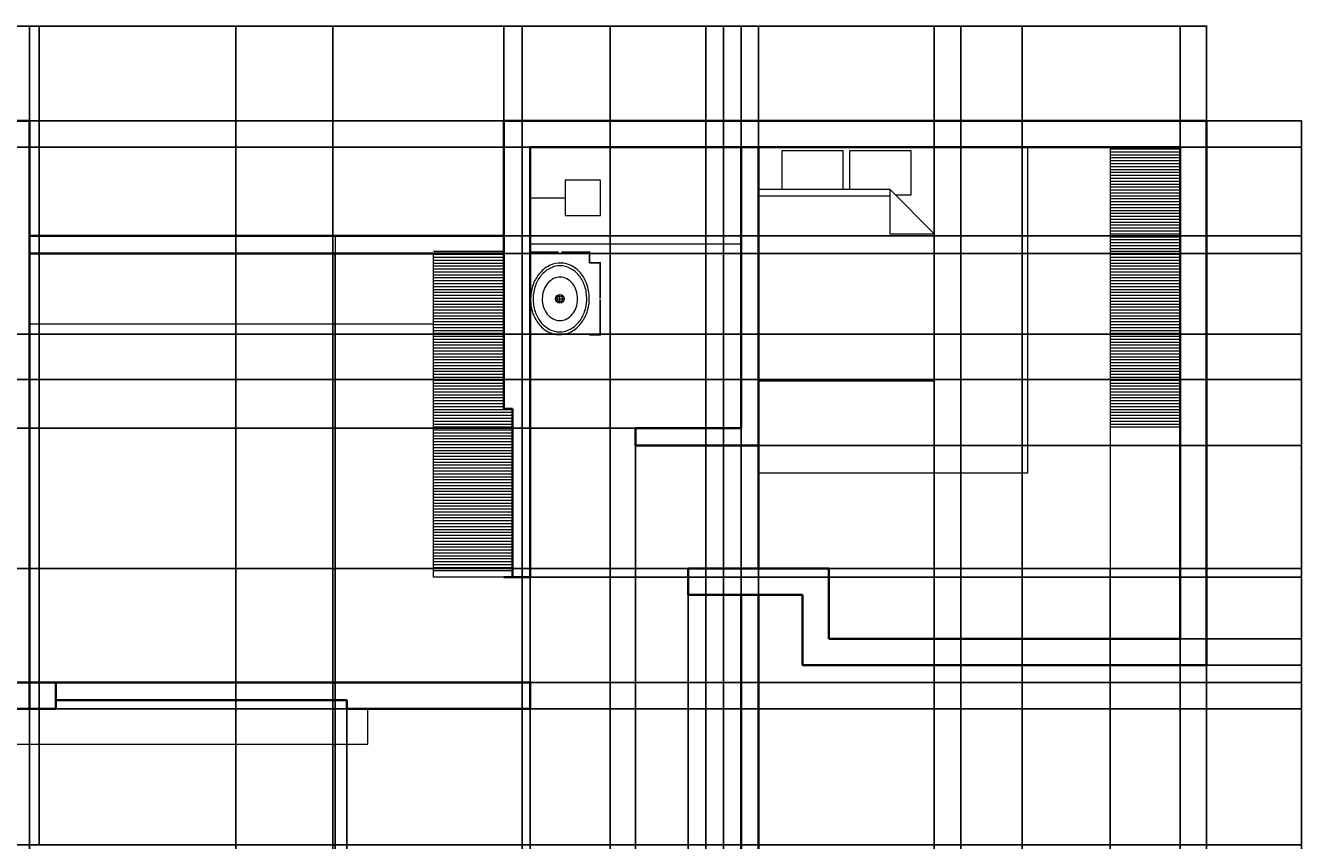
# Model space of a CAD drawing. Units: inches. Extents: x 1159 to 1869, y 2212 to 2738.
# Tile 5 of 5: x 1433 to 1869, y 2460 to 2738. Entities that reach past the tile are written whole.
import ezdxf

# ---------------------------------------------------------------- set-up
doc = ezdxf.new("R2010")
doc.units = ezdxf.units.IN
for name, color, linetype, lineweight in [('A-ANNO-DIMS', 2, 'Continuous', 18), ('A-FLOR', 9, 'Continuous', 13), ('A-FLOR-CASE', 30, 'Continuous', 18), ('A-FLOR-FIXT', 9, 'Continuous', 18), ('A-FLOR-PATT', 252, 'Continuous', 13), ('A-FURN', 8, 'Continuous', 18), ('A-GLAZ', 4, 'Continuous', 18), ('A-WALL', 7, 'Continuous', 35)]:
    doc.layers.add(name, color=color, linetype=linetype, lineweight=lineweight)
doc.styles.get("Standard").update_dxf_attribs({"font": 'arial.ttf'})
doc.dimstyles.get("Standard").update_dxf_attribs({"dimtxt": 0.18, "dimasz": 0.18, "dimexe": 0.18, "dimexo": 0.0625, "dimgap": 0.09, "dimtad": 0, "dimtih": 1, "dimtoh": 1, "dimdec": 4, "dimzin": 0, "dimdsep": 46, "dimtxsty": 'Standard', "dimcen": 0.09, "dimadec": 0, "dimazin": 0, "dimtfac": 1, "dimtdec": 4, "dimtofl": 0, "dimtmove": 0, "dimatfit": 3, "dimfxl": 1, "dimtolj": 1, "dimtzin": 0, "dimarcsym": 0})

# ---------------------------------------------------------------- blocks, each defined once
blk = doc.blocks.new('Bed - Queen')
for p, q in [((0, -80.00003), (0, 0)), ((0, 0), (59.99999, 0)), ((59.99999, 0), (59.99999, -80.00003)), ((7.99999, -1.2), (28.79998, -1.2)), ((7.99999, -14.4), (7.99999, -1.2)), ((28.79998, -1.2), (28.79998, -14.4)), ((31.19999, -1.2), (51.99999, -1.2)), ((31.19999, -14.4), (31.19999, -1.2)), ((51.99999, -1.2), (51.99999, -16.4)), ((0, -14.4), (44.8, -14.4)), ((44.8, -16.8), (0, -16.8)), ((59.99999, -29.6), (44.8, -14.4)), ((44.8, -14.4), (44.8, -29.6)), ((51.99999, -16.4), (46.79936, -16.4)), ((44.8, -29.6), (59.99999, -29.6)), ((59.99999, -80.00003), (0, -80.00003))]:
    blk.add_line(p, q)
blk = doc.blocks.new('Sink - Oval top')
for p, q in [((-1, 0), (1, 0)), ((0, 1), (0, -1))]:
    blk.add_line(p, q)
for points in [[(-12.23, 0.39, 0.117634), (-11.46, -3.36, 0.104469), (-8.88, -6.8, 0.090016), (-5.08, -9.07, 0.08192), (-0.32, -10.02, 0.08192), (4.49, -9.38, 0.090016), (8.42, -7.36, 0.104469), (11.22, -4.09, 0.117634), (12.23, -0.39, 0.117634), (11.46, 3.36, 0.104469), (8.88, 6.8, 0.090016), (5.08, 9.07, 0.08192), (0.32, 10.02, 0.08192), (-4.49, 9.38, 0.090016), (-8.42, 7.36, 0.104469), (-11.22, 4.09, 0.117634)], [(-11.29, 0.16, 0.118622), (-10.52, -3.25, 0.104678), (-8.07, -6.36, 0.089562), (-4.54, -8.37, 0.081185), (-0.13, -9.15, 0.081185), (4.3, -8.49, 0.089562), (7.89, -6.58, 0.104678), (10.42, -3.55, 0.118622), (11.29, -0.16, 0.118622), (10.52, 3.25, 0.104678), (8.07, 6.36, 0.089562), (4.54, 8.37, 0.081185), (0.13, 9.15, 0.081185), (-4.3, 8.49, 0.089562), (-7.89, 6.58, 0.104678), (-10.42, 3.55, 0.118622)], [(-7.42, 0.08, 0.118283), (-6.91, -2.17, 0.104607), (-5.29, -4.21, 0.089718), (-2.97, -5.53, 0.081436), (-0.07, -6.04, 0.081436), (2.84, -5.59, 0.089718), (5.2, -4.33, 0.104607), (6.86, -2.32, 0.118283), (7.42, -0.08, 0.118283), (6.91, 2.17, 0.104607), (5.29, 4.21, 0.089718), (2.97, 5.53, 0.081436), (0.07, 6.04, 0.081436), (-2.84, 5.59, 0.089718), (-5.2, 4.33, 0.104607), (-6.86, 2.32, 0.118283)]]:
    blk.add_lwpolyline(points, format="xyb", close=True)
for radius in [1.5, 1]:
    blk.add_circle((0, 0), radius)
blk = doc.blocks.new('SHOWER-HEAD-SQUARE-12IN')
for p, q in [((6, 12), (0, 12)), ((0, 12), (0, 0)), ((12, 12), (6, 12)), ((12, 0), (12, 12)), ((0, 0), (12, 0))]:
    blk.add_line(p, q)
blk = doc.blocks.new('*D8')
at = {"layer": 'A-ANNO-DIMS', "color": 0, "lineweight": -2, "transparency": 16777216}
for p, q in [((1625.69, 2657.04), (1629.49, 2657.04)), ((1629.31, 2656.86), (1629.31, 2644.95)), ((1629.31, 2632.67), (1629.31, 2644.58)), ((1625.69, 2632.49), (1629.49, 2632.49))]:
    blk.add_line(p, q, dxfattribs=at)
at = {"layer": 'A-ANNO-DIMS', "color": 0, "transparency": 16777216}
for points in [[(1629.28, 2656.86), (1629.34, 2656.86), (1629.31, 2657.04)], [(1629.28, 2632.67), (1629.34, 2632.67), (1629.31, 2632.49)]]:
    blk.add_solid(points, dxfattribs=at)
at = {"layer": 'Defpoints', "color": 0, "transparency": 16777216}
for p in [(1625.62, 2657.04), (1629.31, 2657.04), (1625.62, 2632.49)]:
    blk.add_point(p, dxfattribs=at)
at = {"layer": 'A-ANNO-DIMS', "color": 0, "transparency": 16777216, "insert": (1629.31, 2644.77), "char_height": 0.18, "attachment_point": 5}
blk.add_mtext('\\A1;BASIN 25 TYP.', dxfattribs=at)
blk = doc.blocks.new('*D9')
at = {"layer": 'A-ANNO-DIMS', "color": 0, "lineweight": -2, "transparency": 16777216}
for p, q in [((1605.49, 2657.1), (1605.49, 2660.9)), ((1605.67, 2660.72), (1615.03, 2660.72)), ((1625.44, 2660.72), (1616.09, 2660.72)), ((1625.62, 2657.1), (1625.62, 2660.9))]:
    blk.add_line(p, q, dxfattribs=at)
at = {"layer": 'A-ANNO-DIMS', "color": 0, "transparency": 16777216}
for points in [[(1605.67, 2660.75), (1605.67, 2660.69), (1605.49, 2660.72)], [(1625.44, 2660.75), (1625.44, 2660.69), (1625.62, 2660.72)]]:
    blk.add_solid(points, dxfattribs=at)
at = {"layer": 'Defpoints', "color": 0, "transparency": 16777216}
for p in [(1605.49, 2660.72), (1605.49, 2657.04), (1625.62, 2657.04)]:
    blk.add_point(p, dxfattribs=at)
at = {"layer": 'A-ANNO-DIMS', "color": 0, "transparency": 16777216, "insert": (1615.56, 2660.72), "char_height": 0.18, "attachment_point": 5}
blk.add_mtext('\\A1;20 TYP.', dxfattribs=at)
blk = doc.blocks.new('*D20')
at = {"layer": 'A-ANNO-DIMS', "color": 0, "lineweight": -2, "transparency": 16777216}
for p, q in [((1191.4, 2461.27), (1191.4, 2738.15)), ((1191.58, 2737.97), (1513.61, 2737.97)), ((1836.22, 2737.97), (1514.19, 2737.97)), ((1836.4, 2705.69), (1836.4, 2738.15))]:
    blk.add_line(p, q, dxfattribs=at)
at = {"layer": 'A-ANNO-DIMS', "color": 0, "transparency": 16777216}
for points in [[(1191.58, 2738), (1191.58, 2737.94), (1191.4, 2737.97)], [(1836.22, 2738), (1836.22, 2737.94), (1836.4, 2737.97)]]:
    blk.add_solid(points, dxfattribs=at)
at = {"layer": 'Defpoints', "color": 0, "transparency": 16777216}
for p in [(1836.4, 2737.97), (1836.4, 2705.63), (1191.4, 2461.21)]:
    blk.add_point(p, dxfattribs=at)
at = {"layer": 'A-ANNO-DIMS', "color": 0, "transparency": 16777216, "insert": (1513.9, 2737.97), "char_height": 0.18, "attachment_point": 5}
blk.add_mtext('\\A1;645', dxfattribs=at)
blk = doc.blocks.new('*D21')
at = {"layer": 'A-ANNO-DIMS', "color": 0, "lineweight": -2, "transparency": 16777216}
for p, q in [((1836.46, 2705.63), (1868.92, 2705.63)), ((1868.74, 2705.45), (1868.74, 2475.03)), ((1868.74, 2244.26), (1868.74, 2474.67)), ((1752.46, 2244.08), (1868.92, 2244.08))]:
    blk.add_line(p, q, dxfattribs=at)
at = {"layer": 'A-ANNO-DIMS', "color": 0, "transparency": 16777216}
for points in [[(1868.71, 2705.45), (1868.77, 2705.45), (1868.74, 2705.63)], [(1868.71, 2244.26), (1868.77, 2244.26), (1868.74, 2244.08)]]:
    blk.add_solid(points, dxfattribs=at)
at = {"layer": 'Defpoints', "color": 0, "transparency": 16777216}
for p in [(1836.4, 2705.63), (1868.74, 2705.63), (1752.4, 2244.08)]:
    blk.add_point(p, dxfattribs=at)
at = {"layer": 'A-ANNO-DIMS', "color": 0, "transparency": 16777216, "insert": (1868.74, 2474.85), "char_height": 0.18, "attachment_point": 5}
blk.add_mtext('\\A1;461.55', dxfattribs=at)
blk = doc.blocks.new('*D24')
at = {"layer": 'A-ANNO-DIMS', "color": 0, "lineweight": -2, "transparency": 16777216}
for p, q in [((1434.4, 2666.32), (1434.4, 2738.15)), ((1434.58, 2737.97), (1515.12, 2737.97)), ((1596.22, 2737.97), (1515.68, 2737.97)), ((1596.4, 2666.32), (1596.4, 2738.15))]:
    blk.add_line(p, q, dxfattribs=at)
at = {"layer": 'A-ANNO-DIMS', "color": 0, "transparency": 16777216}
for points in [[(1434.58, 2738), (1434.58, 2737.94), (1434.4, 2737.97)], [(1596.22, 2738), (1596.22, 2737.94), (1596.4, 2737.97)]]:
    blk.add_solid(points, dxfattribs=at)
at = {"layer": 'Defpoints', "color": 0, "transparency": 16777216}
for p in [(1596.4, 2737.97), (1434.4, 2666.26), (1596.4, 2666.26)]:
    blk.add_point(p, dxfattribs=at)
at = {"layer": 'A-ANNO-DIMS', "color": 0, "transparency": 16777216, "insert": (1515.4, 2737.97), "char_height": 0.18, "attachment_point": 5}
blk.add_mtext('\\A1;162', dxfattribs=at)
blk = doc.blocks.new('*D25')
at = {"layer": 'A-ANNO-DIMS', "color": 0, "lineweight": -2, "transparency": 16777216}
for p, q in [((1683.4, 2552.69), (1683.4, 2738.15)), ((1683.58, 2737.97), (1755.12, 2737.97)), ((1827.22, 2737.97), (1755.68, 2737.97)), ((1827.4, 2552.69), (1827.4, 2738.15))]:
    blk.add_line(p, q, dxfattribs=at)
at = {"layer": 'A-ANNO-DIMS', "color": 0, "transparency": 16777216}
for points in [[(1683.58, 2738), (1683.58, 2737.94), (1683.4, 2737.97)], [(1827.22, 2738), (1827.22, 2737.94), (1827.4, 2737.97)]]:
    blk.add_solid(points, dxfattribs=at)
at = {"layer": 'Defpoints', "color": 0, "transparency": 16777216}
for p in [(1827.4, 2737.97), (1683.4, 2552.63), (1827.4, 2552.63)]:
    blk.add_point(p, dxfattribs=at)
at = {"layer": 'A-ANNO-DIMS', "color": 0, "transparency": 16777216, "insert": (1755.4, 2737.97), "char_height": 0.18, "attachment_point": 5}
blk.add_mtext('\\A1;144', dxfattribs=at)
blk = doc.blocks.new('*D31')
at = {"layer": 'A-ANNO-DIMS', "color": 0, "lineweight": -2, "transparency": 16777216}
for p, q in [((1698.46, 2519.63), (1868.92, 2519.63)), ((1868.74, 2519.45), (1868.74, 2484.03)), ((1868.74, 2448.26), (1868.74, 2483.67)), ((1683.46, 2448.08), (1868.92, 2448.08))]:
    blk.add_line(p, q, dxfattribs=at)
at = {"layer": 'A-ANNO-DIMS', "color": 0, "transparency": 16777216}
for points in [[(1868.71, 2519.45), (1868.77, 2519.45), (1868.74, 2519.63)], [(1868.71, 2448.26), (1868.77, 2448.26), (1868.74, 2448.08)]]:
    blk.add_solid(points, dxfattribs=at)
at = {"layer": 'Defpoints', "color": 0, "transparency": 16777216}
for p in [(1698.4, 2519.63), (1683.4, 2448.08), (1868.74, 2448.08)]:
    blk.add_point(p, dxfattribs=at)
at = {"layer": 'A-ANNO-DIMS', "color": 0, "transparency": 16777216, "insert": (1868.74, 2483.85), "char_height": 0.18, "attachment_point": 5}
blk.add_mtext('\\A1;71.55', dxfattribs=at)
blk = doc.blocks.new('*D32')
at = {"layer": 'A-ANNO-DIMS', "color": 0, "lineweight": -2, "transparency": 16777216}
for p, q in [((1743.46, 2696.63), (1868.92, 2696.63)), ((1868.74, 2696.45), (1868.74, 2612.81)), ((1868.74, 2528.81), (1868.74, 2612.45)), ((1707.46, 2528.63), (1868.92, 2528.63))]:
    blk.add_line(p, q, dxfattribs=at)
at = {"layer": 'A-ANNO-DIMS', "color": 0, "transparency": 16777216}
for points in [[(1868.71, 2696.45), (1868.77, 2696.45), (1868.74, 2696.63)], [(1868.71, 2528.81), (1868.77, 2528.81), (1868.74, 2528.63)]]:
    blk.add_solid(points, dxfattribs=at)
at = {"layer": 'Defpoints', "color": 0, "transparency": 16777216}
for p in [(1743.4, 2696.63), (1868.74, 2696.63), (1707.4, 2528.63)]:
    blk.add_point(p, dxfattribs=at)
at = {"layer": 'A-ANNO-DIMS', "color": 0, "transparency": 16777216, "insert": (1868.74, 2612.63), "char_height": 0.18, "attachment_point": 5}
blk.add_mtext('\\A1;168', dxfattribs=at)
blk = doc.blocks.new('*D36')
at = {"layer": 'A-ANNO-DIMS', "color": 0, "lineweight": -2, "transparency": 16777216}
for p, q in [((1752.4, 2337.14), (1752.4, 2738.15)), ((1752.58, 2737.97), (1762.7, 2737.97)), ((1773.22, 2737.97), (1763.1, 2737.97)), ((1773.4, 2343.14), (1773.4, 2738.15))]:
    blk.add_line(p, q, dxfattribs=at)
at = {"layer": 'A-ANNO-DIMS', "color": 0, "transparency": 16777216}
for points in [[(1752.58, 2738), (1752.58, 2737.94), (1752.4, 2737.97)], [(1773.22, 2738), (1773.22, 2737.94), (1773.4, 2737.97)]]:
    blk.add_solid(points, dxfattribs=at)
at = {"layer": 'Defpoints', "color": 0, "transparency": 16777216}
for p in [(1773.4, 2737.97), (1773.4, 2343.08), (1752.4, 2337.08)]:
    blk.add_point(p, dxfattribs=at)
at = {"layer": 'A-ANNO-DIMS', "color": 0, "transparency": 16777216, "insert": (1762.9, 2737.97), "char_height": 0.18, "attachment_point": 5}
blk.add_mtext('\\A1;21', dxfattribs=at)
blk = doc.blocks.new('*D37')
at = {"layer": 'A-ANNO-DIMS', "color": 0, "lineweight": -2, "transparency": 16777216}
for p, q in [((1434.46, 2705.63), (1868.92, 2705.63)), ((1868.74, 2705.45), (1868.74, 2686.13)), ((1868.74, 2666.44), (1868.74, 2685.76)), ((1434.46, 2666.26), (1868.92, 2666.26))]:
    blk.add_line(p, q, dxfattribs=at)
at = {"layer": 'A-ANNO-DIMS', "color": 0, "transparency": 16777216}
for points in [[(1868.71, 2705.45), (1868.77, 2705.45), (1868.74, 2705.63)], [(1868.71, 2666.44), (1868.77, 2666.44), (1868.74, 2666.26)]]:
    blk.add_solid(points, dxfattribs=at)
at = {"layer": 'Defpoints', "color": 0, "transparency": 16777216}
for p in [(1434.4, 2705.63), (1868.74, 2705.63), (1434.4, 2666.26)]:
    blk.add_point(p, dxfattribs=at)
at = {"layer": 'A-ANNO-DIMS', "color": 0, "transparency": 16777216, "insert": (1868.74, 2685.94), "char_height": 0.18, "attachment_point": 5}
blk.add_mtext('\\A1;39.37', dxfattribs=at)
blk = doc.blocks.new('*D38')
at = {"layer": 'A-ANNO-DIMS', "color": 0, "lineweight": -2, "transparency": 16777216}
for p, q in [((1434.46, 2660.26), (1868.92, 2660.26)), ((1868.74, 2660.08), (1868.74, 2587.13)), ((1868.74, 2513.81), (1868.74, 2586.76)), ((1443.46, 2513.63), (1868.92, 2513.63))]:
    blk.add_line(p, q, dxfattribs=at)
at = {"layer": 'A-ANNO-DIMS', "color": 0, "transparency": 16777216}
for points in [[(1868.71, 2660.08), (1868.77, 2660.08), (1868.74, 2660.26)], [(1868.71, 2513.81), (1868.77, 2513.81), (1868.74, 2513.63)]]:
    blk.add_solid(points, dxfattribs=at)
at = {"layer": 'Defpoints', "color": 0, "transparency": 16777216}
for p in [(1434.4, 2660.26), (1868.74, 2660.26), (1443.4, 2513.63)]:
    blk.add_point(p, dxfattribs=at)
at = {"layer": 'A-ANNO-DIMS', "color": 0, "transparency": 16777216, "insert": (1868.74, 2586.94), "char_height": 0.18, "attachment_point": 5}
blk.add_mtext('\\A1;146.63', dxfattribs=at)
blk = doc.blocks.new('*D39')
at = {"layer": 'A-ANNO-DIMS', "color": 0, "lineweight": -2, "transparency": 16777216}
for p, q in [((1605.4, 2696.57), (1605.4, 2211.56)), ((1677.4, 2696.57), (1677.4, 2211.56)), ((1605.58, 2211.74), (1641.18, 2211.74)), ((1677.22, 2211.74), (1641.62, 2211.74))]:
    blk.add_line(p, q, dxfattribs=at)
at = {"layer": 'A-ANNO-DIMS', "color": 0, "transparency": 16777216}
for points in [[(1605.58, 2211.77), (1605.58, 2211.71), (1605.4, 2211.74)], [(1677.22, 2211.77), (1677.22, 2211.71), (1677.4, 2211.74)]]:
    blk.add_solid(points, dxfattribs=at)
at = {"layer": 'Defpoints', "color": 0, "transparency": 16777216}
for p in [(1605.4, 2696.63), (1677.4, 2696.63), (1677.4, 2211.74)]:
    blk.add_point(p, dxfattribs=at)
at = {"layer": 'A-ANNO-DIMS', "color": 0, "transparency": 16777216, "insert": (1641.4, 2211.74), "char_height": 0.18, "attachment_point": 5}
blk.add_mtext('\\A1;72', dxfattribs=at)
blk = doc.blocks.new('*D40')
at = {"layer": 'A-ANNO-DIMS', "color": 0, "lineweight": -2, "transparency": 16777216}
for p, q in [((1677.34, 2696.63), (1158.88, 2696.63)), ((1159.06, 2696.45), (1159.06, 2648.81)), ((1159.06, 2600.81), (1159.06, 2648.45)), ((1677.34, 2600.63), (1158.88, 2600.63))]:
    blk.add_line(p, q, dxfattribs=at)
at = {"layer": 'A-ANNO-DIMS', "color": 0, "transparency": 16777216}
for points in [[(1159.03, 2696.45), (1159.09, 2696.45), (1159.06, 2696.63)], [(1159.03, 2600.81), (1159.09, 2600.81), (1159.06, 2600.63)]]:
    blk.add_solid(points, dxfattribs=at)
at = {"layer": 'Defpoints', "color": 0, "transparency": 16777216}
for p in [(1159.06, 2696.63), (1677.4, 2696.63), (1677.4, 2600.63)]:
    blk.add_point(p, dxfattribs=at)
at = {"layer": 'A-ANNO-DIMS', "color": 0, "transparency": 16777216, "insert": (1159.06, 2648.63), "char_height": 0.18, "attachment_point": 5}
blk.add_mtext('\\A1;96', dxfattribs=at)
blk = doc.blocks.new('*D43')
at = {"layer": 'A-ANNO-DIMS', "color": 0, "lineweight": -2, "transparency": 16777216}
for p, q in [((1671.4, 2439.14), (1671.4, 2738.15)), ((1671.58, 2737.97), (1707.18, 2737.97)), ((1743.22, 2737.97), (1707.62, 2737.97)), ((1743.4, 2439.14), (1743.4, 2738.15))]:
    blk.add_line(p, q, dxfattribs=at)
at = {"layer": 'A-ANNO-DIMS', "color": 0, "transparency": 16777216}
for points in [[(1671.58, 2738), (1671.58, 2737.94), (1671.4, 2737.97)], [(1743.22, 2738), (1743.22, 2737.94), (1743.4, 2737.97)]]:
    blk.add_solid(points, dxfattribs=at)
at = {"layer": 'Defpoints', "color": 0, "transparency": 16777216}
for p in [(1743.4, 2737.97), (1671.4, 2439.08), (1743.4, 2439.08)]:
    blk.add_point(p, dxfattribs=at)
at = {"layer": 'A-ANNO-DIMS', "color": 0, "transparency": 16777216, "insert": (1707.4, 2737.97), "char_height": 0.18, "attachment_point": 5}
blk.add_mtext('\\A1;72', dxfattribs=at)
blk = doc.blocks.new('*D47')
at = {"layer": 'A-ANNO-DIMS', "color": 0, "lineweight": -2, "transparency": 16777216}
for p, q in [((1605.46, 2549.63), (1868.92, 2549.63)), ((1868.74, 2549.45), (1868.74, 2531.81)), ((1868.74, 2513.81), (1868.74, 2531.45)), ((1605.46, 2513.63), (1868.92, 2513.63))]:
    blk.add_line(p, q, dxfattribs=at)
at = {"layer": 'A-ANNO-DIMS', "color": 0, "transparency": 16777216}
for points in [[(1868.71, 2549.45), (1868.77, 2549.45), (1868.74, 2549.63)], [(1868.71, 2513.81), (1868.77, 2513.81), (1868.74, 2513.63)]]:
    blk.add_solid(points, dxfattribs=at)
at = {"layer": 'Defpoints', "color": 0, "transparency": 16777216}
for p in [(1605.4, 2549.63), (1605.4, 2513.63), (1868.74, 2513.63)]:
    blk.add_point(p, dxfattribs=at)
at = {"layer": 'A-ANNO-DIMS', "color": 0, "transparency": 16777216, "insert": (1868.74, 2531.63), "char_height": 0.18, "attachment_point": 5}
blk.add_mtext('\\A1;36', dxfattribs=at)
blk = doc.blocks.new('*D48')
at = {"layer": 'A-ANNO-DIMS', "color": 0, "lineweight": -2, "transparency": 16777216}
for p, q in [((1437.74, 2458.27), (1437.74, 2738.15)), ((1437.92, 2737.97), (1519.76, 2737.97)), ((1602.5, 2737.97), (1520.67, 2737.97)), ((1602.68, 2448.14), (1602.68, 2738.15))]:
    blk.add_line(p, q, dxfattribs=at)
at = {"layer": 'A-ANNO-DIMS', "color": 0, "transparency": 16777216}
for points in [[(1437.92, 2738), (1437.92, 2737.94), (1437.74, 2737.97)], [(1602.5, 2738), (1602.5, 2737.94), (1602.68, 2737.97)]]:
    blk.add_solid(points, dxfattribs=at)
at = {"layer": 'Defpoints', "color": 0, "transparency": 16777216}
for p in [(1602.68, 2737.97), (1437.74, 2458.21), (1602.68, 2448.08)]:
    blk.add_point(p, dxfattribs=at)
at = {"layer": 'A-ANNO-DIMS', "color": 0, "transparency": 16777216, "insert": (1520.21, 2737.97), "char_height": 0.18, "attachment_point": 5}
blk.add_mtext('\\A1;164.94', dxfattribs=at)
blk = doc.blocks.new('*D53')
at = {"layer": 'A-ANNO-DIMS', "color": 0, "lineweight": -2, "transparency": 16777216}
for p, q in [((1425.46, 2504.63), (1868.92, 2504.63)), ((1868.74, 2504.45), (1868.74, 2481.6)), ((1868.74, 2458.39), (1868.74, 2481.24)), ((1428.81, 2458.21), (1868.92, 2458.21))]:
    blk.add_line(p, q, dxfattribs=at)
at = {"layer": 'A-ANNO-DIMS', "color": 0, "transparency": 16777216}
for points in [[(1868.71, 2504.45), (1868.77, 2504.45), (1868.74, 2504.63)], [(1868.71, 2458.39), (1868.77, 2458.39), (1868.74, 2458.21)]]:
    blk.add_solid(points, dxfattribs=at)
at = {"layer": 'Defpoints', "color": 0, "transparency": 16777216}
for p in [(1425.4, 2504.63), (1868.74, 2504.63), (1428.74, 2458.21)]:
    blk.add_point(p, dxfattribs=at)
at = {"layer": 'A-ANNO-DIMS', "color": 0, "transparency": 16777216, "insert": (1868.74, 2481.42), "char_height": 0.18, "attachment_point": 5}
blk.add_mtext('\\A1;46.42', dxfattribs=at)
blk = doc.blocks.new('*D57')
at = {"layer": 'A-ANNO-DIMS', "color": 0, "lineweight": -2, "transparency": 16777216}
for p, q in [((1504.87, 2433.16), (1504.87, 2738.15)), ((1505.05, 2737.97), (1521.04, 2737.97)), ((1537.79, 2737.97), (1521.8, 2737.97)), ((1537.97, 2433.16), (1537.97, 2738.15))]:
    blk.add_line(p, q, dxfattribs=at)
at = {"layer": 'A-ANNO-DIMS', "color": 0, "transparency": 16777216}
for points in [[(1505.05, 2738), (1505.05, 2737.94), (1504.87, 2737.97)], [(1537.79, 2738), (1537.79, 2737.94), (1537.97, 2737.97)]]:
    blk.add_solid(points, dxfattribs=at)
at = {"layer": 'Defpoints', "color": 0, "transparency": 16777216}
for p in [(1537.97, 2737.97), (1504.87, 2433.09), (1537.97, 2433.09)]:
    blk.add_point(p, dxfattribs=at)
at = {"layer": 'A-ANNO-DIMS', "color": 0, "transparency": 16777216, "insert": (1521.42, 2737.97), "char_height": 0.18, "attachment_point": 5}
blk.add_mtext('\\A1;33.11', dxfattribs=at)
blk = doc.blocks.new('*D60')
at = {"layer": 'A-ANNO-DIMS', "color": 0, "lineweight": -2, "transparency": 16777216}
for p, q in [((1659.4, 2552.57), (1659.4, 2211.56)), ((1605.4, 2549.57), (1605.4, 2211.56)), ((1605.58, 2211.74), (1632.18, 2211.74)), ((1659.22, 2211.74), (1632.62, 2211.74))]:
    blk.add_line(p, q, dxfattribs=at)
at = {"layer": 'A-ANNO-DIMS', "color": 0, "transparency": 16777216}
for points in [[(1605.58, 2211.77), (1605.58, 2211.71), (1605.4, 2211.74)], [(1659.22, 2211.77), (1659.22, 2211.71), (1659.4, 2211.74)]]:
    blk.add_solid(points, dxfattribs=at)
at = {"layer": 'Defpoints', "color": 0, "transparency": 16777216}
for p in [(1659.4, 2552.63), (1605.4, 2549.63), (1605.4, 2211.74)]:
    blk.add_point(p, dxfattribs=at)
at = {"layer": 'A-ANNO-DIMS', "color": 0, "transparency": 16777216, "insert": (1632.4, 2211.74), "char_height": 0.18, "attachment_point": 5}
blk.add_mtext('\\A1;54', dxfattribs=at)
blk = doc.blocks.new('*D61')
at = {"layer": 'A-ANNO-DIMS', "color": 0, "lineweight": -2, "transparency": 16777216}
for p, q in [((1632.68, 2448.14), (1632.68, 2738.15)), ((1632.86, 2737.97), (1648.65, 2737.97)), ((1665.22, 2737.97), (1649.43, 2737.97)), ((1665.4, 2448.14), (1665.4, 2738.15))]:
    blk.add_line(p, q, dxfattribs=at)
at = {"layer": 'A-ANNO-DIMS', "color": 0, "transparency": 16777216}
for points in [[(1632.86, 2738), (1632.86, 2737.94), (1632.68, 2737.97)], [(1665.22, 2738), (1665.22, 2737.94), (1665.4, 2737.97)]]:
    blk.add_solid(points, dxfattribs=at)
at = {"layer": 'Defpoints', "color": 0, "transparency": 16777216}
for p in [(1665.4, 2737.97), (1632.68, 2448.08), (1665.4, 2448.08)]:
    blk.add_point(p, dxfattribs=at)
at = {"layer": 'A-ANNO-DIMS', "color": 0, "transparency": 16777216, "insert": (1649.04, 2737.97), "char_height": 0.18, "attachment_point": 5}
blk.add_mtext('\\A1;32.72', dxfattribs=at)
blk = doc.blocks.new('*D64')
at = {"layer": 'A-ANNO-DIMS', "color": 0, "lineweight": -2, "transparency": 16777216}
for p, q in [((1434.4, 2660.2), (1434.4, 2211.56)), ((1538.82, 2660.2), (1538.82, 2211.56)), ((1434.58, 2211.74), (1486.15, 2211.74)), ((1538.64, 2211.74), (1487.06, 2211.74))]:
    blk.add_line(p, q, dxfattribs=at)
at = {"layer": 'A-ANNO-DIMS', "color": 0, "transparency": 16777216}
for points in [[(1434.58, 2211.77), (1434.58, 2211.71), (1434.4, 2211.74)], [(1538.64, 2211.77), (1538.64, 2211.71), (1538.82, 2211.74)]]:
    blk.add_solid(points, dxfattribs=at)
at = {"layer": 'Defpoints', "color": 0, "transparency": 16777216}
for p in [(1434.4, 2660.26), (1538.82, 2660.26), (1434.4, 2211.74)]:
    blk.add_point(p, dxfattribs=at)
at = {"layer": 'A-ANNO-DIMS', "color": 0, "transparency": 16777216, "insert": (1486.61, 2211.74), "char_height": 0.18, "attachment_point": 5}
blk.add_mtext('\\A1;104.42', dxfattribs=at)
blk = doc.blocks.new('*D65')
at = {"layer": 'A-ANNO-DIMS', "color": 0, "lineweight": -2, "transparency": 16777216}
for p, q in [((1542.76, 2504.57), (1542.76, 2211.56)), ((1605.4, 2504.57), (1605.4, 2211.56)), ((1542.94, 2211.74), (1573.69, 2211.74)), ((1605.22, 2211.74), (1574.48, 2211.74))]:
    blk.add_line(p, q, dxfattribs=at)
at = {"layer": 'A-ANNO-DIMS', "color": 0, "transparency": 16777216}
for points in [[(1542.94, 2211.77), (1542.94, 2211.71), (1542.76, 2211.74)], [(1605.22, 2211.77), (1605.22, 2211.71), (1605.4, 2211.74)]]:
    blk.add_solid(points, dxfattribs=at)
at = {"layer": 'Defpoints', "color": 0, "transparency": 16777216}
for p in [(1542.76, 2504.63), (1605.4, 2504.63), (1605.4, 2211.74)]:
    blk.add_point(p, dxfattribs=at)
at = {"layer": 'A-ANNO-DIMS', "color": 0, "transparency": 16777216, "insert": (1574.08, 2211.74), "char_height": 0.18, "attachment_point": 5}
blk.add_mtext('\\A1;62.64', dxfattribs=at)
blk = doc.blocks.new('*D66')
at = {"layer": 'A-ANNO-DIMS', "color": 0, "lineweight": -2, "transparency": 16777216}
for p, q in [((1605.4, 2696.57), (1605.4, 2211.56)), ((1641.4, 2600.57), (1641.4, 2211.56)), ((1605.58, 2211.74), (1623.18, 2211.74)), ((1641.22, 2211.74), (1623.62, 2211.74))]:
    blk.add_line(p, q, dxfattribs=at)
at = {"layer": 'A-ANNO-DIMS', "color": 0, "transparency": 16777216}
for points in [[(1605.58, 2211.77), (1605.58, 2211.71), (1605.4, 2211.74)], [(1641.22, 2211.77), (1641.22, 2211.71), (1641.4, 2211.74)]]:
    blk.add_solid(points, dxfattribs=at)
at = {"layer": 'Defpoints', "color": 0, "transparency": 16777216}
for p in [(1605.4, 2696.63), (1641.4, 2600.63), (1605.4, 2211.74)]:
    blk.add_point(p, dxfattribs=at)
at = {"layer": 'A-ANNO-DIMS', "color": 0, "transparency": 16777216, "insert": (1623.4, 2211.74), "char_height": 0.18, "attachment_point": 5}
blk.add_mtext('\\A1;36', dxfattribs=at)
blk = doc.blocks.new('*D68')
at = {"layer": 'A-ANNO-DIMS', "color": 0, "lineweight": -2, "transparency": 16777216}
for p, q in [((1803.4, 2552.57), (1803.4, 2211.56)), ((1827.4, 2552.57), (1827.4, 2211.56)), ((1803.58, 2211.74), (1815.18, 2211.74)), ((1827.22, 2211.74), (1815.62, 2211.74))]:
    blk.add_line(p, q, dxfattribs=at)
at = {"layer": 'A-ANNO-DIMS', "color": 0, "transparency": 16777216}
for points in [[(1803.58, 2211.77), (1803.58, 2211.71), (1803.4, 2211.74)], [(1827.22, 2211.77), (1827.22, 2211.71), (1827.4, 2211.74)]]:
    blk.add_solid(points, dxfattribs=at)
at = {"layer": 'Defpoints', "color": 0, "transparency": 16777216}
for p in [(1803.4, 2552.63), (1827.4, 2552.63), (1827.4, 2211.74)]:
    blk.add_point(p, dxfattribs=at)
at = {"layer": 'A-ANNO-DIMS', "color": 0, "transparency": 16777216, "insert": (1815.4, 2211.74), "char_height": 0.18, "attachment_point": 5}
blk.add_mtext('\\A1;24', dxfattribs=at)
blk = doc.blocks.new('*D69')
at = {"layer": 'A-ANNO-DIMS', "color": 0, "lineweight": -2, "transparency": 16777216}
for p, q in [((1803.34, 2696.63), (1158.88, 2696.63)), ((1159.06, 2696.45), (1159.06, 2624.81)), ((1159.06, 2552.81), (1159.06, 2624.45)), ((1803.34, 2552.63), (1158.88, 2552.63))]:
    blk.add_line(p, q, dxfattribs=at)
at = {"layer": 'A-ANNO-DIMS', "color": 0, "transparency": 16777216}
for points in [[(1159.03, 2696.45), (1159.09, 2696.45), (1159.06, 2696.63)], [(1159.03, 2552.81), (1159.09, 2552.81), (1159.06, 2552.63)]]:
    blk.add_solid(points, dxfattribs=at)
at = {"layer": 'Defpoints', "color": 0, "transparency": 16777216}
for p in [(1159.06, 2696.63), (1803.4, 2696.63), (1803.4, 2552.63)]:
    blk.add_point(p, dxfattribs=at)
at = {"layer": 'A-ANNO-DIMS', "color": 0, "transparency": 16777216, "insert": (1159.06, 2624.63), "char_height": 0.18, "attachment_point": 5}
blk.add_mtext('\\A1;144', dxfattribs=at)
blk = doc.blocks.new('*D70')
at = {"layer": 'A-ANNO-DIMS', "color": 0, "lineweight": -2, "transparency": 16777216}
for p, q in [((1827.4, 2528.57), (1827.4, 2211.56)), ((1836.4, 2519.57), (1836.4, 2211.56)), ((1827.58, 2211.74), (1831.75, 2211.74)), ((1836.22, 2211.74), (1832.05, 2211.74))]:
    blk.add_line(p, q, dxfattribs=at)
at = {"layer": 'A-ANNO-DIMS', "color": 0, "transparency": 16777216}
for points in [[(1827.58, 2211.77), (1827.58, 2211.71), (1827.4, 2211.74)], [(1836.22, 2211.77), (1836.22, 2211.71), (1836.4, 2211.74)]]:
    blk.add_solid(points, dxfattribs=at)
at = {"layer": 'Defpoints', "color": 0, "transparency": 16777216}
for p in [(1827.4, 2528.63), (1836.4, 2519.63), (1836.4, 2211.74)]:
    blk.add_point(p, dxfattribs=at)
at = {"layer": 'A-ANNO-DIMS', "color": 0, "transparency": 16777216, "insert": (1831.9, 2211.74), "char_height": 0.18, "attachment_point": 5}
blk.add_mtext('\\A1;9', dxfattribs=at)
blk = doc.blocks.new('*D71')
at = {"layer": 'A-ANNO-DIMS', "color": 0, "lineweight": -2, "transparency": 16777216}
for p, q in [((1677.4, 2448.14), (1677.4, 2738.15)), ((1677.58, 2737.97), (1680.25, 2737.97)), ((1683.22, 2737.97), (1680.55, 2737.97)), ((1683.4, 2448.14), (1683.4, 2738.15))]:
    blk.add_line(p, q, dxfattribs=at)
at = {"layer": 'A-ANNO-DIMS', "color": 0, "transparency": 16777216}
for points in [[(1677.58, 2738), (1677.58, 2737.94), (1677.4, 2737.97)], [(1683.22, 2738), (1683.22, 2737.94), (1683.4, 2737.97)]]:
    blk.add_solid(points, dxfattribs=at)
at = {"layer": 'Defpoints', "color": 0, "transparency": 16777216}
for p in [(1683.4, 2737.97), (1677.4, 2448.08), (1683.4, 2448.08)]:
    blk.add_point(p, dxfattribs=at)
at = {"layer": 'A-ANNO-DIMS', "color": 0, "transparency": 16777216, "insert": (1680.4, 2737.97), "char_height": 0.18, "attachment_point": 5}
blk.add_mtext('\\A1;6', dxfattribs=at)
blk = doc.blocks.new('*D73')
at = {"layer": 'A-ANNO-DIMS', "color": 0, "lineweight": -2, "transparency": 16777216}
for p, q in [((1303.3, 2632.72), (1868.92, 2632.72)), ((1868.74, 2632.54), (1868.74, 2625.14)), ((1868.74, 2617.39), (1868.74, 2624.78)), ((1305.46, 2617.21), (1868.92, 2617.21))]:
    blk.add_line(p, q, dxfattribs=at)
at = {"layer": 'A-ANNO-DIMS', "color": 0, "transparency": 16777216}
for points in [[(1868.71, 2632.54), (1868.77, 2632.54), (1868.74, 2632.72)], [(1868.71, 2617.39), (1868.77, 2617.39), (1868.74, 2617.21)]]:
    blk.add_solid(points, dxfattribs=at)
at = {"layer": 'Defpoints', "color": 0, "transparency": 16777216}
for p in [(1303.24, 2632.72), (1868.74, 2632.72), (1305.4, 2617.21)]:
    blk.add_point(p, dxfattribs=at)
at = {"layer": 'A-ANNO-DIMS', "color": 0, "transparency": 16777216, "insert": (1868.74, 2624.96), "char_height": 0.18, "attachment_point": 5}
blk.add_mtext('\\A1;15.51', dxfattribs=at)
blk = doc.blocks.new('*D76')
at = {"layer": 'A-ANNO-DIMS', "color": 0, "lineweight": -2, "transparency": 16777216}
for p, q in [((1683.46, 2594.63), (1868.92, 2594.63)), ((1868.74, 2594.45), (1868.74, 2573.81)), ((1868.74, 2552.81), (1868.74, 2573.45)), ((1683.46, 2552.63), (1868.92, 2552.63))]:
    blk.add_line(p, q, dxfattribs=at)
at = {"layer": 'A-ANNO-DIMS', "color": 0, "transparency": 16777216}
for points in [[(1868.71, 2594.45), (1868.77, 2594.45), (1868.74, 2594.63)], [(1868.71, 2552.81), (1868.77, 2552.81), (1868.74, 2552.63)]]:
    blk.add_solid(points, dxfattribs=at)
at = {"layer": 'Defpoints', "color": 0, "transparency": 16777216}
for p in [(1683.4, 2594.63), (1868.74, 2594.63), (1683.4, 2552.63)]:
    blk.add_point(p, dxfattribs=at)
at = {"layer": 'A-ANNO-DIMS', "color": 0, "transparency": 16777216, "insert": (1868.74, 2573.63), "char_height": 0.18, "attachment_point": 5}
blk.add_mtext('\\A1;42', dxfattribs=at)

msp = doc.modelspace()

# ---------------------------------------------------------------- hatches: boundary and pattern name
at = {"layer": 'A-FLOR-PATT'}
h = msp.add_hatch(dxfattribs=at)
h.set_pattern_fill('ANSI31', color=256, scale=0.3149606, angle=-45, style=0)
h.paths.add_polyline_path([(1803.4011, 2600.1922), (1827.4011, 2600.1922), (1827.4011, 2696.6279), (1803.4011, 2696.6279)])
h = msp.add_hatch(dxfattribs=at)
h.set_pattern_fill('ANSI31', color=256, scale=0.3149606, angle=-45, style=0)
h.paths.add_polyline_path([(1572.4011, 2551.0403), (1599.4011, 2551.0403), (1599.4011, 2607.1472), (1596.4011, 2607.1472), (1596.4011, 2661.0403), (1572.4011, 2661.0403)])

# ---------------------------------------------------------------- linework, layer by layer
at = {"layer": 'A-FLOR'}
for p, q in [((1775.1775, 2696.6279), (1775.1775, 2585.1564)), ((1775.1775, 2585.1564), (1683.4011, 2585.1564))]:
    msp.add_line(p, q, dxfattribs=at)
at = {"layer": 'A-FLOR-CASE'}
for p, q in [((1803.4011, 2696.6279), (1803.4011, 2552.6279)), ((1572.4011, 2549.6279), (1572.4011, 2660.2597)), ((1434.4011, 2636.2597), (1572.4011, 2636.2597)), ((1827.4011, 2552.6279), (1707.4011, 2552.6279)), ((1596.4011, 2549.6279), (1572.4011, 2549.6279)), ((1549.9486, 2492.6279), (1549.9486, 2504.6279)), ((1425.4011, 2492.6279), (1549.9486, 2492.6279))]:
    msp.add_line(p, q, dxfattribs=at)
at = {"layer": 'A-FLOR-FIXT'}
for p, q in [((1605.4011, 2679.2793), (1617.4011, 2679.2793)), ((1605.4011, 2663.5619), (1677.4011, 2663.5619))]:
    msp.add_line(p, q, dxfattribs=at)
at = {"layer": 'A-GLAZ'}
msp.add_line((1538.817, 2666.2597), (1538.817, 2660.2597), dxfattribs=at)
at = {"layer": 'A-WALL'}
for p, q in [((1272.4011, 2705.6279), (1434.4011, 2705.6279)), ((1434.4011, 2705.6279), (1434.4011, 2504.6279)), ((1596.4011, 2607.1472), (1596.4011, 2705.6279)), ((1596.4011, 2705.6279), (1836.4011, 2705.6279)), ((1836.4011, 2705.6279), (1836.4011, 2552.6279)), ((1605.4011, 2696.6279), (1677.4011, 2696.6279)), ((1605.4011, 2549.6279), (1605.4011, 2696.6279)), ((1677.4011, 2696.6279), (1683.4011, 2696.6279)), ((1677.4011, 2696.6279), (1677.4011, 2624.6279)), ((1683.4011, 2696.6279), (1827.4011, 2696.6279)), ((1683.4011, 2696.6279), (1683.4011, 2624.6279)), ((1827.4011, 2696.6279), (1827.4011, 2552.6279)), ((1434.4011, 2666.2597), (1596.4011, 2666.2597)), ((1434.4011, 2660.2597), (1596.4011, 2660.2597)), ((1677.4011, 2624.6279), (1677.4011, 2600.6279)), ((1683.4011, 2624.6279), (1683.4011, 2594.6279)), ((1599.4011, 2607.1472), (1596.4011, 2607.1472)), ((1599.4011, 2549.6279), (1599.4011, 2607.1472)), ((1677.4011, 2600.6279), (1641.4011, 2600.6279)), ((1641.4011, 2594.6279), (1641.4011, 2600.6279)), ((1683.4011, 2594.6279), (1641.4011, 2594.6279)), ((1683.4011, 2594.6279), (1683.4011, 2552.6279)), ((1707.4011, 2552.6279), (1659.4011, 2552.6279)), ((1659.4011, 2552.6279), (1659.4011, 2543.6279)), ((1707.4011, 2540.6279), (1707.4011, 2552.6279)), ((1827.4011, 2552.6279), (1827.4011, 2528.6279)), ((1836.4011, 2552.6279), (1836.4011, 2519.6279)), ((1596.4011, 2549.6279), (1605.4011, 2549.6279)), ((1596.4011, 2549.6279), (1599.4011, 2549.6279)), ((1659.4011, 2543.6279), (1698.4011, 2543.6279)), ((1677.4011, 2543.6279), (1677.4011, 2448.0757)), ((1683.4011, 2543.6279), (1683.4011, 2448.0757)), ((1698.4011, 2543.6279), (1698.4011, 2540.6279)), ((1698.4011, 2519.6279), (1698.4011, 2540.6279)), ((1707.4011, 2528.6279), (1707.4011, 2540.6279)), ((1827.4011, 2528.6279), (1707.4011, 2528.6279)), ((1836.4011, 2519.6279), (1698.4011, 2519.6279)), ((1425.4011, 2513.6279), (1569.4011, 2513.6279)), ((1443.4011, 2504.6279), (1443.4011, 2513.6279)), ((1569.4011, 2513.6279), (1605.4011, 2513.6279)), ((1605.4011, 2504.6279), (1605.4011, 2513.6279)), ((1443.4011, 2504.6279), (1443.4011, 2507.6279)), ((1443.4011, 2507.6279), (1542.764, 2507.6279)), ((1542.764, 2507.6279), (1542.764, 2504.6279)), ((1425.4011, 2504.6279), (1443.4011, 2504.6279)), ((1434.4011, 2504.6279), (1443.4011, 2504.6279)), ((1542.764, 2504.6279), (1569.4011, 2504.6279)), ((1569.4011, 2504.6279), (1605.4011, 2504.6279))]:
    msp.add_line(p, q, dxfattribs=at)

# ---------------------------------------------------------------- block references
at = {"layer": 'A-FLOR-FIXT'}
for name, p, rotation in [('SHOWER-HEAD-SQUARE-12IN', (1629.4008, 2673.279), 89.99999999999895), ('Sink - Oval top', (1615.5557, 2644.7657), 90)]:
    msp.add_blockref(name, p, dxfattribs=dict(at, rotation=rotation))
at = {"layer": 'A-FURN'}
msp.add_blockref('Bed - Queen', (1683.4011, 2696.6279), dxfattribs=at)

# ---------------------------------------------------------------- dimensions: what is measured, and where the dimension line sits
at = {"layer": 'A-ANNO-DIMS'}
for base, p1, p2, override, picture, middle in [((1836.4011, 2737.9679), (1191.4011, 2461.2064), (1836.4011, 2705.6279), {"dimdec": 0, "dimlfac": 1, "dimrnd": 0, "dimzin": 0, "dimdsep": 46, "dimlunit": 2}, '*D20', (1513.9011, 2737.9679)), ((1596.4011, 2737.9679), (1434.4011, 2666.2597), (1596.4011, 2666.2597), {"dimdec": 0, "dimlfac": 1, "dimrnd": 0, "dimzin": 0, "dimdsep": 46, "dimlunit": 2}, '*D24', (1515.4011, 2737.9679)), ((1602.6806, 2737.9679), (1437.7443, 2458.2064), (1602.6806, 2448.0757), {"dimdec": 2, "dimlfac": 1, "dimrnd": 0, "dimzin": 0, "dimdsep": 46, "dimlunit": 2}, '*D48', (1520.2124, 2737.9679)), ((1537.9722, 2737.9679), (1504.8654, 2433.0936), (1537.9722, 2433.0936), {"dimdec": 2, "dimlfac": 1, "dimrnd": 0, "dimzin": 0, "dimdsep": 46, "dimlunit": 2}, '*D57', (1521.4188, 2737.9679)), ((1665.4011, 2737.9679), (1632.6806, 2448.0757), (1665.4011, 2448.0757), {"dimdec": 2, "dimlfac": 1, "dimrnd": 0, "dimzin": 0, "dimdsep": 46, "dimlunit": 2}, '*D61', (1649.0408, 2737.9679)), ((1743.4011, 2737.9679), (1671.4011, 2439.0757), (1743.4011, 2439.0757), {"dimdec": 0, "dimlfac": 1, "dimrnd": 0, "dimzin": 0, "dimdsep": 46, "dimlunit": 2}, '*D43', (1707.4011, 2737.9679)), ((1683.4011, 2737.9679), (1677.4011, 2448.0757), (1683.4011, 2448.0757), {"dimdec": 0, "dimlfac": 1, "dimrnd": 0, "dimzin": 0, "dimdsep": 46, "dimlunit": 2}, '*D71', (1680.4011, 2737.9679)), ((1827.4011, 2737.9679), (1683.4011, 2552.6279), (1827.4011, 2552.6279), {"dimdec": 0, "dimlfac": 1, "dimrnd": 0, "dimzin": 0, "dimdsep": 46, "dimlunit": 2}, '*D25', (1755.4011, 2737.9679)), ((1773.4011, 2737.9679), (1752.4011, 2337.0757), (1773.4011, 2343.0757), {"dimdec": 0, "dimlfac": 1, "dimrnd": 0, "dimzin": 0, "dimdsep": 46, "dimlunit": 2}, '*D36', (1762.9011, 2737.9679)), ((1677.4011, 2211.7357), (1605.4011, 2696.6279), (1677.4011, 2696.6279), {"dimdec": 0, "dimlfac": 1, "dimrnd": 0, "dimzin": 0, "dimdsep": 46, "dimlunit": 2}, '*D39', (1641.4011, 2211.7357)), ((1605.4011, 2211.7357), (1641.4011, 2600.6279), (1605.4011, 2696.6279), {"dimdec": 0, "dimlfac": 1, "dimrnd": 0, "dimzin": 0, "dimdsep": 46, "dimlunit": 2}, '*D66', (1623.4011, 2211.7357)), ((1434.4011, 2211.7357), (1538.817, 2660.2597), (1434.4011, 2660.2597), {"dimdec": 2, "dimlfac": 1, "dimrnd": 0, "dimzin": 0, "dimdsep": 46, "dimlunit": 2}, '*D64', (1486.6091, 2211.7357)), ((1605.4011, 2211.7357), (1659.4011, 2552.6279), (1605.4011, 2549.6279), {"dimdec": 0, "dimlfac": 1, "dimrnd": 0, "dimzin": 0, "dimdsep": 46, "dimlunit": 2}, '*D60', (1632.4011, 2211.7357)), ((1827.4011, 2211.7357), (1803.4011, 2552.6279), (1827.4011, 2552.6279), {"dimdec": 0, "dimlfac": 1, "dimrnd": 0, "dimzin": 0, "dimdsep": 46, "dimlunit": 2}, '*D68', (1815.4011, 2211.7357)), ((1836.4011, 2211.7357), (1827.4011, 2528.6279), (1836.4011, 2519.6279), {"dimdec": 0, "dimlfac": 1, "dimrnd": 0, "dimzin": 0, "dimdsep": 46, "dimlunit": 2}, '*D70', (1831.9011, 2211.7357)), ((1605.4011, 2211.7357), (1542.764, 2504.6279), (1605.4011, 2504.6279), {"dimdec": 2, "dimlfac": 1, "dimrnd": 0, "dimzin": 0, "dimdsep": 46, "dimlunit": 2}, '*D65', (1574.0826, 2211.7357))]:
    dim = msp.add_linear_dim(base=base, p1=p1, p2=p2, dimstyle='Standard', override=override, dxfattribs=at)
    dim.commit()
    dim.dimension.update_dxf_attribs({"geometry": picture, "text_midpoint": middle})
for base, p1, p2, override, picture, middle in [((1868.7411, 2705.6279), (1434.4011, 2666.2597), (1434.4011, 2705.6279), {"dimdec": 2, "dimlfac": 1, "dimrnd": 0, "dimzin": 0, "dimdsep": 46, "dimlunit": 2}, '*D37', (1868.7411, 2685.9438)), ((1868.7411, 2705.6279), (1752.4011, 2244.0757), (1836.4011, 2705.6279), {"dimdec": 2, "dimlfac": 1, "dimrnd": 0, "dimzin": 0, "dimdsep": 46, "dimlunit": 2}, '*D21', (1868.7411, 2474.8518)), ((1159.0611, 2696.6279), (1803.4011, 2552.6279), (1803.4011, 2696.6279), {"dimdec": 0, "dimlfac": 1, "dimrnd": 0, "dimzin": 0, "dimdsep": 46, "dimlunit": 2}, '*D69', (1159.0611, 2624.6279)), ((1159.0611, 2696.6279), (1677.4011, 2600.6279), (1677.4011, 2696.6279), {"dimdec": 0, "dimlfac": 1, "dimrnd": 0, "dimzin": 0, "dimdsep": 46, "dimlunit": 2}, '*D40', (1159.0611, 2648.6279)), ((1868.7411, 2696.6279), (1707.4011, 2528.6279), (1743.4011, 2696.6279), {"dimdec": 0, "dimlfac": 1, "dimrnd": 0, "dimzin": 0, "dimdsep": 46, "dimlunit": 2}, '*D32', (1868.7411, 2612.6279)), ((1868.7411, 2660.2597), (1443.4011, 2513.6279), (1434.4011, 2660.2597), {"dimdec": 2, "dimlfac": 1, "dimrnd": 0, "dimzin": 0, "dimdsep": 46, "dimlunit": 2}, '*D38', (1868.7411, 2586.9438)), ((1868.7411, 2632.7174), (1305.4011, 2617.2064), (1303.2377, 2632.7174), {"dimdec": 2, "dimlfac": 1, "dimrnd": 0, "dimzin": 0, "dimdsep": 46, "dimlunit": 2}, '*D73', (1868.7411, 2624.9619)), ((1868.7411, 2594.6279), (1683.4011, 2552.6279), (1683.4011, 2594.6279), {"dimdec": 0, "dimlfac": 1, "dimrnd": 0, "dimzin": 0, "dimdsep": 46, "dimlunit": 2}, '*D76', (1868.7411, 2573.6279)), ((1868.7411, 2513.6279), (1605.4011, 2549.6279), (1605.4011, 2513.6279), {"dimdec": 0, "dimlfac": 1, "dimrnd": 0, "dimzin": 0, "dimdsep": 46, "dimlunit": 2}, '*D47', (1868.7411, 2531.6279)), ((1868.7411, 2448.0757), (1698.4011, 2519.6279), (1683.4011, 2448.0757), {"dimdec": 2, "dimlfac": 1, "dimrnd": 0, "dimzin": 0, "dimdsep": 46, "dimlunit": 2}, '*D31', (1868.7411, 2483.8518)), ((1868.7411, 2504.6279), (1428.7443, 2458.2064), (1425.4011, 2504.6279), {"dimdec": 2, "dimlfac": 1, "dimrnd": 0, "dimzin": 0, "dimdsep": 46, "dimlunit": 2}, '*D53', (1868.7411, 2481.4172))]:
    dim = msp.add_linear_dim(base=base, p1=p1, p2=p2, angle=90, dimstyle='Standard', override=override, dxfattribs=at)
    dim.commit()
    dim.dimension.update_dxf_attribs({"geometry": picture, "text_midpoint": middle})
for base, p1, p2, angle, text, picture, middle in [((1605.4874, 2660.7238), (1625.624, 2657.0411), (1605.4874, 2657.0411), 180, '<> TYP.', '*D9', (1615.5557, 2660.7238)), ((1629.3067, 2657.0411), (1625.624, 2632.4902), (1625.624, 2657.0411), 90, 'BASIN <> TYP.', '*D8', (1629.3067, 2644.7657))]:
    dim = msp.add_linear_dim(base=base, p1=p1, p2=p2, angle=angle, text=text, dimstyle='Standard', override={"dimdec": 0, "dimlfac": 1, "dimrnd": 0, "dimzin": 0, "dimdsep": 46, "dimlunit": 2}, dxfattribs=at)
    dim.commit()
    dim.dimension.update_dxf_attribs({"geometry": picture, "text_midpoint": middle})

doc.saveas('drawing.dxf')
